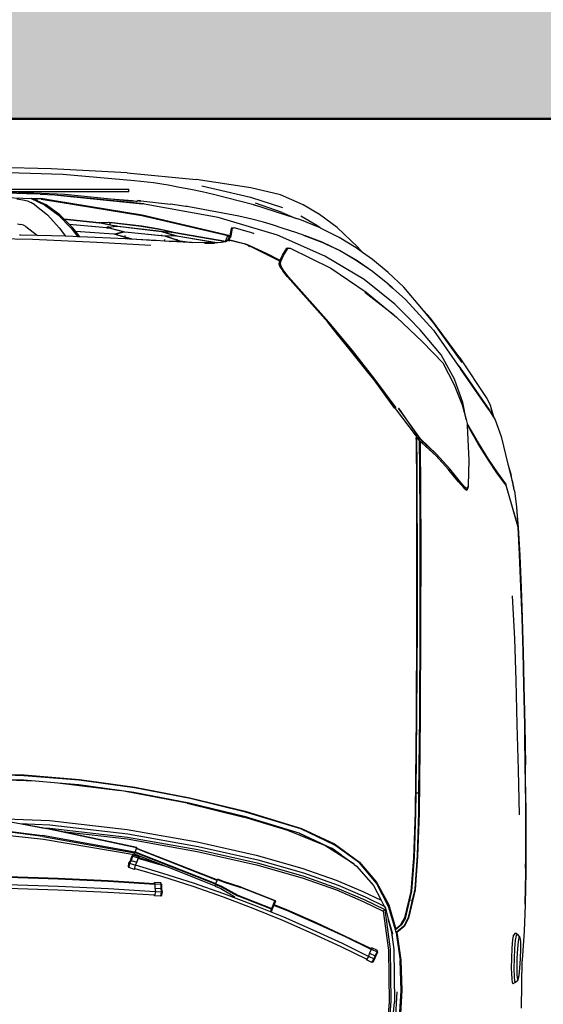
# Model space of a CAD drawing. Units: inches. Extents: x 22042254 to 25404563, y 17568978 to 17626777.
# Tile 34 of 45: x 22179853 to 22179890, y 17626332 to 17626402. Entities that reach past the tile are written whole.
import ezdxf

# ---------------------------------------------------------------- set-up
doc = ezdxf.new("R2010")
doc.units = ezdxf.units.IN
doc.header["$MEASUREMENT"] = 0
for name, color, linetype, lineweight in [('A-SITE-VEHI', 8, 'Continuous', 18), ('A-WALL-PATT', 244, 'Continuous', 13), ('walls', 252, 'Continuous', 50)]:
    doc.layers.add(name, color=color, linetype=linetype, lineweight=lineweight)
doc.layers.add('Edges', color=250, linetype='Continuous')

# ---------------------------------------------------------------- blocks, each defined once
blk = doc.blocks.new('Nissan Qashqai pl')
at = {"layer": 'Edges'}
for p, q in [((7.8676, 12.8123), (7.7998, 12.7928)), ((7.8012, 12.7929), (7.8681, 12.8121)), ((7.8363, 12.8097), (7.8676, 12.8123)), ((7.8381, 12.81), (7.87, 12.8126)), ((7.8676, 12.8123), (7.8681, 12.8121)), ((7.869, 12.8124), (7.8681, 12.8121)), ((7.9137, 12.815), (7.869, 12.8124)), ((7.87, 12.8126), (7.9151, 12.8152)), ((7.9658, 12.8172), (7.9137, 12.815)), ((7.9151, 12.8152), (7.9668, 12.8174)), ((8.016, 12.8189), (7.9658, 12.8172)), ((7.9668, 12.8174), (8.0168, 12.8191)), ((8.0713, 12.8205), (8.016, 12.8189)), ((8.0168, 12.8191), (8.0718, 12.8207)), ((8.1249, 12.8218), (8.0713, 12.8205)), ((8.0718, 12.8207), (8.1251, 12.822)), ((8.1901, 12.8232), (8.1249, 12.8218)), ((8.1251, 12.822), (8.1902, 12.8233)), ((8.1888, 12.8107), (8.2622, 12.8125)), ((8.2094, 12.8235), (8.1901, 12.8232)), ((8.1902, 12.8233), (8.2543, 12.8243)), ((8.2543, 12.8243), (8.2094, 12.8235)), ((8.2543, 12.8243), (8.2094, 12.8235)), ((8.2544, 12.8242), (8.2094, 12.8235)), ((8.2693, 12.8245), (8.2543, 12.8243)), ((8.3166, 12.8249), (8.2544, 12.8242)), ((8.2622, 12.8125), (8.3356, 12.8141)), ((8.3098, 12.825), (8.2693, 12.8245)), ((8.3159, 12.825), (8.2693, 12.8245)), ((8.3159, 12.825), (8.3098, 12.825)), ((8.3159, 12.825), (8.3163, 12.825)), ((8.3163, 12.825), (8.3657, 12.8252)), ((8.3163, 12.825), (8.3597, 12.8252)), ((8.3764, 12.8251), (8.3166, 12.8249)), ((8.3597, 12.8252), (8.3657, 12.8252)), ((8.3657, 12.8252), (8.3663, 12.8252)), ((8.3663, 12.8252), (8.3747, 12.8252)), ((8.3764, 12.8251), (8.3663, 12.8252)), ((8.3747, 12.8252), (8.3757, 12.8252)), ((8.3757, 12.8252), (8.4282, 12.8249)), ((8.4069, 12.8249), (8.3764, 12.8251)), ((8.4219, 12.8246), (8.4069, 12.8249)), ((8.4292, 12.8248), (8.4069, 12.8249)), ((8.4282, 12.8249), (8.4799, 12.8239)), ((8.4799, 12.8239), (8.4292, 12.8248)), ((8.4799, 12.8239), (8.4811, 12.8239)), ((8.4811, 12.8239), (8.5241, 12.8222)), ((8.5241, 12.8222), (8.5707, 12.8193)), ((8.5287, 12.8112), (8.5331, 12.815)), ((8.5347, 12.8159), (8.5331, 12.815)), ((8.5331, 12.815), (8.5346, 12.8138)), ((8.5346, 12.8138), (8.5406, 12.8125)), ((8.5407, 12.8167), (8.5347, 12.8159)), ((8.5406, 12.8125), (8.5526, 12.8114)), ((8.5527, 12.8169), (8.5407, 12.8167)), ((8.5682, 12.8164), (8.5527, 12.8169)), ((8.5837, 12.8154), (8.5682, 12.8164)), ((8.5707, 12.8193), (8.5719, 12.8193)), ((8.6489, 12.8179), (8.5719, 12.8193)), ((8.5958, 12.8141), (8.5837, 12.8154)), ((8.6018, 12.8129), (8.5958, 12.8141)), ((8.6017, 12.8114), (8.6032, 12.8121)), ((8.6032, 12.8121), (8.6018, 12.8129)), ((8.6073, 12.808), (8.6032, 12.8121)), ((7.7223, 12.7851), (7.7673, 12.7961)), ((7.7673, 12.7961), (7.8058, 12.8055)), ((7.7673, 12.7961), (7.7848, 12.8012)), ((7.7835, 12.8007), (7.7835, 12.8007)), ((7.8087, 12.8062), (7.7848, 12.8012)), ((7.7865, 12.8013), (7.7866, 12.8013)), ((7.7936, 12.8029), (7.7977, 12.8038)), ((7.8106, 12.8065), (7.8087, 12.8062)), ((7.8106, 12.8065), (7.8107, 12.8065)), ((7.8107, 12.8065), (7.8363, 12.8097)), ((7.8363, 12.8097), (7.8381, 12.81)), ((7.9803, 12.803), (8.05, 12.8066)), ((8.05, 12.8066), (8.1176, 12.8087)), ((8.1176, 12.8087), (8.1888, 12.8107)), ((8.5287, 12.8112), (8.5269, 12.8082)), ((8.5322, 12.8047), (8.5269, 12.8082)), ((8.5287, 12.8112), (8.531, 12.8095)), ((8.531, 12.8095), (8.5385, 12.8079)), ((8.5322, 12.8047), (8.5375, 12.8036)), ((8.5375, 12.8036), (8.5513, 12.8023)), ((8.5385, 12.8079), (8.5518, 12.8066)), ((8.5513, 12.8023), (8.5678, 12.8016)), ((8.5518, 12.8066), (8.568, 12.8059)), ((8.5526, 12.8114), (8.5681, 12.8107)), ((8.5678, 12.8016), (8.5844, 12.8014)), ((8.568, 12.8059), (8.5842, 12.8057)), ((8.5681, 12.8107), (8.5836, 12.8104)), ((8.5836, 12.8104), (8.5957, 12.8107)), ((8.5842, 12.8057), (8.5974, 12.8061)), ((8.5844, 12.8014), (8.5921, 12.8016)), ((8.5921, 12.8016), (8.6021, 12.8022)), ((8.5957, 12.8107), (8.6017, 12.8114)), ((8.5974, 12.8061), (8.6049, 12.8069)), ((8.6021, 12.8022), (8.6065, 12.8027)), ((8.6049, 12.8069), (8.6073, 12.808)), ((8.6065, 12.8027), (8.6093, 12.804)), ((8.6073, 12.808), (8.6093, 12.804)), ((7.6953, 12.7753), (7.7223, 12.7851)), ((7.7814, 12.7791), (7.7991, 12.7923)), ((7.7984, 12.7909), (7.7828, 12.7793)), ((7.7976, 12.792), (7.7991, 12.7923)), ((7.8007, 12.7926), (7.7984, 12.7909)), ((7.7991, 12.7923), (7.7998, 12.7928)), ((7.7995, 12.7924), (7.8007, 12.7926)), ((7.8012, 12.7929), (7.8007, 12.7926)), ((7.6799, 12.7658), (7.6125, 12.719)), ((7.6608, 12.7617), (7.6712, 12.7675)), ((7.6712, 12.7675), (7.6721, 12.7679)), ((7.6926, 12.7737), (7.6721, 12.7679)), ((7.6759, 12.7633), (7.6793, 12.7657)), ((7.6911, 12.7728), (7.6774, 12.7688)), ((7.6793, 12.7657), (7.6802, 12.766)), ((7.6799, 12.7658), (7.6802, 12.766)), ((7.6802, 12.766), (7.6809, 12.7664)), ((7.6809, 12.7664), (7.6911, 12.7728)), ((7.6911, 12.7728), (7.6926, 12.7737)), ((7.6926, 12.7737), (7.6953, 12.7753)), ((7.7325, 12.7476), (7.7591, 12.7641)), ((7.7606, 12.7644), (7.7341, 12.7478)), ((7.7591, 12.7641), (7.7814, 12.7791)), ((7.7828, 12.7793), (7.7606, 12.7644)), ((7.5946, 12.718), (7.6608, 12.7617)), ((7.6113, 12.7186), (7.6759, 12.7633)), ((7.7341, 12.7478), (7.7056, 12.7314)), ((7.7038, 12.731), (7.7325, 12.7476)), ((7.7048, 12.7302), (7.7608, 12.7329)), ((7.7608, 12.7329), (7.8014, 12.7318)), ((7.7688, 12.7328), (7.7688, 12.734)), ((7.5946, 12.718), (7.5304, 12.6704)), ((7.6024, 12.7221), (7.5387, 12.6759)), ((7.6051, 12.7139), (7.6113, 12.7186)), ((7.6051, 12.7139), (7.6111, 12.7181)), ((7.6118, 12.7186), (7.6111, 12.7181)), ((7.6125, 12.719), (7.6118, 12.7186)), ((7.667, 12.723), (7.6295, 12.7097)), ((7.6386, 12.7089), (7.6708, 12.7217)), ((7.6949, 12.7283), (7.667, 12.723)), ((7.6708, 12.7217), (7.6949, 12.7283)), ((7.6949, 12.7283), (7.701, 12.73)), ((7.701, 12.73), (7.7024, 12.7301)), ((7.7024, 12.7301), (7.7038, 12.731)), ((7.7024, 12.7301), (7.7034, 12.7301)), ((7.7056, 12.7314), (7.7034, 12.7301)), ((7.7034, 12.7301), (7.7048, 12.7302)), ((7.7058, 12.7308), (7.7048, 12.7302)), ((7.7938, 12.7171), (7.7748, 12.7018)), ((7.7959, 12.7161), (7.7772, 12.7011)), ((7.8045, 12.7263), (7.7938, 12.7171)), ((7.8062, 12.725), (7.7959, 12.7161)), ((7.8014, 12.7318), (7.8022, 12.7316)), ((7.8022, 12.7316), (7.8037, 12.7315)), ((7.8022, 12.7316), (7.8072, 12.73)), ((7.8037, 12.7315), (7.8096, 12.7294)), ((7.8072, 12.73), (7.8045, 12.7263)), ((7.8062, 12.725), (7.8087, 12.7283)), ((7.8066, 12.7254), (7.8062, 12.725)), ((7.8096, 12.7294), (7.8066, 12.7254)), ((7.8072, 12.73), (7.8087, 12.7283)), ((7.5501, 12.6757), (7.6051, 12.7139)), ((7.6295, 12.7097), (7.59, 12.6877)), ((7.6032, 12.6908), (7.6386, 12.7089)), ((7.7748, 12.7018), (7.7507, 12.6803)), ((7.7772, 12.7011), (7.776, 12.6999)), ((7.59, 12.6877), (7.5492, 12.654)), ((7.5687, 12.6579), (7.6032, 12.6908)), ((7.753, 12.6794), (7.776, 12.6999)), ((7.776, 12.6999), (7.7539, 12.68)), ((7.5501, 12.6757), (7.5001, 12.6302)), ((7.5387, 12.6759), (7.5184, 12.6591)), ((7.5184, 12.6591), (7.5304, 12.6704)), ((7.7261, 12.6543), (7.7507, 12.6803)), ((7.753, 12.6794), (7.7281, 12.6524)), ((7.7507, 12.6803), (7.7286, 12.6561)), ((7.7539, 12.68), (7.7324, 12.6565)), ((7.5184, 12.6591), (7.4801, 12.6274)), ((7.5289, 12.6158), (7.5687, 12.6579)), ((7.5492, 12.654), (7.531, 12.6359)), ((7.7261, 12.6543), (7.6762, 12.6186)), ((7.7281, 12.6524), (7.7232, 12.6486)), ((7.7267, 12.6539), (7.7233, 12.6514)), ((7.7286, 12.6561), (7.7267, 12.6539)), ((7.7299, 12.6537), (7.7281, 12.6524)), ((7.7281, 12.6524), (7.7349, 12.6524)), ((7.7324, 12.6565), (7.7299, 12.6537)), ((7.7299, 12.6537), (7.7334, 12.6537)), ((7.7334, 12.6537), (7.8083, 12.6544)), ((7.7349, 12.6524), (7.768, 12.6527)), ((7.768, 12.6527), (7.7692, 12.6527)), ((7.7692, 12.6527), (7.7844, 12.6528)), ((7.7844, 12.6528), (7.8078, 12.653)), ((7.8078, 12.653), (7.8233, 12.6531)), ((7.8083, 12.6544), (7.904, 12.6547)), ((7.8233, 12.6531), (7.9036, 12.6534)), ((7.9036, 12.6534), (8.0275, 12.6533)), ((7.904, 12.6547), (8.0276, 12.6545)), ((8.0275, 12.6533), (8.1755, 12.6527)), ((8.0276, 12.6545), (8.1753, 12.6539)), ((8.1753, 12.6539), (8.3324, 12.6521)), ((8.1755, 12.6527), (8.3005, 12.6514)), ((8.3324, 12.6521), (8.4022, 12.6498)), ((7.6762, 12.6186), (7.7233, 12.6514)), ((7.6771, 12.6135), (7.7215, 12.6473)), ((7.7215, 12.6473), (7.7221, 12.6478)), ((7.7232, 12.6486), (7.7221, 12.6478)), ((7.7245, 12.6486), (7.7232, 12.6486)), ((7.7261, 12.6476), (7.7238, 12.6476)), ((7.7294, 12.6487), (7.7245, 12.6486)), ((7.7279, 12.6477), (7.7261, 12.6476)), ((7.8048, 12.6483), (7.7279, 12.6477)), ((7.731, 12.6487), (7.7294, 12.6487)), ((7.764, 12.6489), (7.731, 12.6487)), ((7.7662, 12.6489), (7.764, 12.6489)), ((7.7811, 12.649), (7.7662, 12.6489)), ((7.7822, 12.649), (7.7811, 12.649)), ((7.8057, 12.6491), (7.7822, 12.649)), ((7.9014, 12.6487), (7.8048, 12.6483)), ((7.8233, 12.6492), (7.8057, 12.6491)), ((7.902, 12.6495), (7.8233, 12.6492)), ((8.0273, 12.6485), (7.9014, 12.6487)), ((8.0275, 12.6493), (7.902, 12.6495)), ((8.1753, 12.6479), (8.0273, 12.6485)), ((8.1754, 12.6487), (8.0275, 12.6493)), ((8.3318, 12.6462), (8.1753, 12.6479)), ((8.3002, 12.6474), (8.1754, 12.6487)), ((8.3005, 12.6514), (8.3002, 12.6474)), ((8.332, 12.6471), (8.3002, 12.6474)), ((8.3005, 12.6514), (8.3324, 12.651)), ((8.4049, 12.6437), (8.3318, 12.6462)), ((8.4042, 12.6447), (8.332, 12.6471)), ((8.3324, 12.651), (8.4014, 12.6488)), ((8.4014, 12.6488), (8.4559, 12.6451)), ((8.4022, 12.6498), (8.4571, 12.6459)), ((8.4588, 12.6405), (8.4042, 12.6447)), ((8.4595, 12.6395), (8.4049, 12.6437)), ((8.4559, 12.6451), (8.4736, 12.6409)), ((8.4571, 12.6459), (8.5029, 12.635)), ((8.4729, 12.6372), (8.4588, 12.6405)), ((8.5025, 12.6293), (8.4595, 12.6395)), ((8.4729, 12.6372), (8.4736, 12.6409)), ((8.5032, 12.6301), (8.4729, 12.6372)), ((8.4736, 12.6409), (8.5018, 12.6344)), ((7.4801, 12.6274), (7.4565, 12.6023)), ((7.4827, 12.6103), (7.5001, 12.6302)), ((7.531, 12.6359), (7.5081, 12.6131)), ((7.531, 12.6359), (7.5301, 12.6353)), ((8.5018, 12.6344), (8.5155, 12.6274)), ((8.5125, 12.6231), (8.5025, 12.6293)), ((8.5029, 12.635), (8.5163, 12.6279)), ((8.5132, 12.624), (8.5032, 12.6301)), ((8.5177, 12.617), (8.5125, 12.6231)), ((8.5132, 12.624), (8.5216, 12.6139)), ((8.5155, 12.6274), (8.5258, 12.6151)), ((8.5163, 12.6279), (8.5237, 12.6189)), ((8.5294, 12.6167), (8.5706, 12.6226)), ((8.5304, 12.6157), (8.5715, 12.6215)), ((8.5706, 12.6226), (8.6197, 12.6241)), ((8.6203, 12.6229), (8.5715, 12.6215)), ((8.6197, 12.6241), (8.6683, 12.6215)), ((8.6203, 12.6229), (8.6204, 12.6229)), ((8.6721, 12.6201), (8.6204, 12.6229)), ((7.5081, 12.6131), (7.4679, 12.5634)), ((7.4744, 12.6015), (7.4804, 12.6079)), ((7.4762, 12.6028), (7.478, 12.6049)), ((7.4804, 12.6079), (7.478, 12.6049)), ((7.478, 12.6049), (7.479, 12.6061)), ((7.479, 12.6061), (7.4815, 12.6089)), ((7.479, 12.6061), (7.4801, 12.6074)), ((7.4801, 12.6074), (7.4804, 12.6079)), ((7.4804, 12.6079), (7.4807, 12.6082)), ((7.4804, 12.6079), (7.4804, 12.6079)), ((7.4807, 12.6082), (7.4821, 12.6097)), ((7.4815, 12.6089), (7.4821, 12.6097)), ((7.4821, 12.6097), (7.4827, 12.6103)), ((7.4882, 12.5645), (7.5243, 12.6101)), ((7.4884, 12.5664), (7.5289, 12.6158)), ((7.5243, 12.6101), (7.5286, 12.6146)), ((7.676, 12.6152), (7.6296, 12.5803)), ((7.6769, 12.6129), (7.6306, 12.5791)), ((8.4814, 12.6029), (8.5166, 12.6135)), ((8.5216, 12.6139), (8.4838, 12.6027)), ((8.4889, 12.5969), (8.5531, 12.6055)), ((8.5039, 12.6023), (8.528, 12.6088)), ((8.5216, 12.6068), (8.5039, 12.6023)), ((8.5166, 12.6135), (8.5197, 12.6145)), ((8.5197, 12.6145), (8.5177, 12.617)), ((8.5197, 12.6145), (8.5216, 12.6139)), ((8.5258, 12.6151), (8.5216, 12.6139)), ((8.5216, 12.6068), (8.5538, 12.6111)), ((8.5301, 12.609), (8.5216, 12.6068)), ((8.5237, 12.6189), (8.5259, 12.6162)), ((8.5259, 12.6162), (8.5258, 12.6151)), ((8.5258, 12.6151), (8.5304, 12.6157)), ((8.5259, 12.6162), (8.5294, 12.6167)), ((8.5304, 12.6157), (8.5304, 12.6157)), ((8.5531, 12.6055), (8.6375, 12.6066)), ((8.5538, 12.6111), (8.6387, 12.6123)), ((8.622, 12.6161), (8.6699, 12.6132)), ((8.6375, 12.6066), (8.7481, 12.5968)), ((8.6721, 12.6093), (8.6387, 12.6123)), ((7.4565, 12.6023), (7.4354, 12.5766)), ((7.4542, 12.5765), (7.4744, 12.6015)), ((7.475, 12.6016), (7.4549, 12.5767)), ((7.4762, 12.6028), (7.475, 12.6016)), ((7.4752, 12.6016), (7.4762, 12.6028)), ((8.4444, 12.5834), (8.4814, 12.6029)), ((8.4838, 12.6027), (8.4462, 12.5833)), ((8.4499, 12.5782), (8.4737, 12.5908)), ((8.4594, 12.5611), (8.4737, 12.5908)), ((8.468, 12.5648), (8.4831, 12.5957)), ((8.4725, 12.563), (8.4889, 12.5969)), ((8.4737, 12.5908), (8.4831, 12.5957)), ((8.4756, 12.5615), (8.4914, 12.5942)), ((8.4831, 12.5957), (8.4867, 12.5977)), ((8.4867, 12.5977), (8.5039, 12.6023)), ((8.4914, 12.5942), (8.4889, 12.5969)), ((8.4914, 12.5942), (8.5544, 12.6026)), ((8.5544, 12.6026), (8.6386, 12.6037)), ((8.6386, 12.6037), (8.7491, 12.594)), ((7.4354, 12.5766), (7.4239, 12.5604)), ((7.4363, 12.5502), (7.4542, 12.5765)), ((7.4549, 12.5767), (7.4369, 12.5504)), ((7.6296, 12.5803), (7.5827, 12.5441)), ((7.6301, 12.5787), (7.618, 12.5691)), ((7.6306, 12.5791), (7.6301, 12.5787)), ((8.4122, 12.5558), (8.4444, 12.5834)), ((8.4462, 12.5833), (8.4134, 12.5554)), ((8.4183, 12.5508), (8.4499, 12.5782)), ((8.5527, 12.5749), (8.5323, 12.5332)), ((8.5537, 12.5747), (8.5332, 12.5329)), ((8.5554, 12.5847), (8.551, 12.5757)), ((8.5527, 12.5749), (8.551, 12.5757)), ((8.551, 12.5757), (8.5528, 12.5751)), ((8.5528, 12.5751), (8.5527, 12.5749)), ((8.5528, 12.5751), (8.5529, 12.5751)), ((8.5529, 12.5751), (8.5572, 12.5841)), ((8.5529, 12.5751), (8.5537, 12.5747)), ((8.5537, 12.5747), (8.5595, 12.572)), ((8.5574, 12.5849), (8.5554, 12.5847)), ((8.5572, 12.5841), (8.5554, 12.5847)), ((8.5639, 12.581), (8.5572, 12.5841)), ((8.5574, 12.5849), (8.5584, 12.5846)), ((8.5582, 12.5845), (8.5574, 12.5849)), ((8.5584, 12.5846), (8.5649, 12.5816)), ((8.5595, 12.572), (8.5639, 12.581)), ((8.5687, 12.5791), (8.5639, 12.581)), ((8.5644, 12.5701), (8.5687, 12.5791)), ((8.5649, 12.5816), (8.5693, 12.5799)), ((8.5687, 12.5791), (8.5693, 12.5799)), ((8.5749, 12.5757), (8.5687, 12.5791)), ((8.5693, 12.5799), (8.5739, 12.5774)), ((8.5749, 12.5757), (8.5705, 12.5668)), ((8.5739, 12.5774), (8.5749, 12.5757)), ((7.4239, 12.5604), (7.4147, 12.5524)), ((7.4239, 12.5604), (7.4166, 12.5503)), ((7.4679, 12.5634), (7.4302, 12.4993)), ((7.4498, 12.5093), (7.4884, 12.5664)), ((7.618, 12.5691), (7.5829, 12.5411)), ((7.618, 12.5691), (7.584, 12.5429)), ((8.4411, 12.5178), (8.4594, 12.5611)), ((8.4493, 12.5212), (8.468, 12.5648)), ((8.454, 12.5196), (8.4725, 12.563)), ((8.4571, 12.5184), (8.4756, 12.5615)), ((8.5647, 12.57), (8.5441, 12.5279)), ((8.5487, 12.5256), (8.5692, 12.5674)), ((8.5595, 12.572), (8.5644, 12.5701)), ((8.5644, 12.5701), (8.5647, 12.57)), ((8.5647, 12.57), (8.5692, 12.5675)), ((8.5692, 12.5674), (8.5692, 12.5675)), ((8.5692, 12.5675), (8.5705, 12.5668)), ((8.5705, 12.5668), (8.5692, 12.5674)), ((7.4147, 12.5524), (7.3837, 12.5197)), ((7.4166, 12.5503), (7.3997, 12.5227)), ((7.4205, 12.5229), (7.4363, 12.5502)), ((7.4369, 12.5504), (7.4211, 12.5232)), ((7.5827, 12.5441), (7.5369, 12.5057)), ((7.584, 12.5429), (7.5568, 12.5201)), ((7.5829, 12.5411), (7.5568, 12.5201)), ((8.3826, 12.5151), (8.4122, 12.5558)), ((8.4134, 12.5554), (8.3844, 12.5157)), ((8.4154, 12.5468), (8.3852, 12.4994)), ((8.3901, 12.5113), (8.4154, 12.5468)), ((8.4011, 12.5269), (8.4154, 12.5468)), ((8.4156, 12.547), (8.4154, 12.5468)), ((8.4156, 12.547), (8.4183, 12.5508)), ((8.4011, 12.5269), (8.3901, 12.5113)), ((8.3904, 12.512), (8.4011, 12.5269)), ((8.5323, 12.5332), (8.5103, 12.4859)), ((8.5332, 12.5329), (8.5112, 12.4856)), ((8.5441, 12.5279), (8.5222, 12.4807)), ((8.5269, 12.4785), (8.5487, 12.5256)), ((7.3837, 12.5197), (7.3624, 12.4907)), ((7.3997, 12.5227), (7.3845, 12.4925)), ((7.4071, 12.4948), (7.4205, 12.5229)), ((7.4211, 12.5232), (7.4078, 12.4951)), ((7.4172, 12.4431), (7.4498, 12.5093)), ((7.5568, 12.5201), (7.5371, 12.5042)), ((8.3573, 12.4618), (8.3826, 12.5151)), ((8.3844, 12.5157), (8.3582, 12.4606)), ((8.3646, 12.4572), (8.39, 12.5111)), ((8.3648, 12.4579), (8.39, 12.5111)), ((8.39, 12.5111), (8.3852, 12.4994)), ((8.39, 12.5111), (8.3901, 12.5113)), ((8.3901, 12.5113), (8.3904, 12.512)), ((8.4217, 12.4622), (8.4411, 12.5178)), ((8.4296, 12.4651), (8.4493, 12.5212)), ((8.4343, 12.4637), (8.454, 12.5196)), ((8.4375, 12.4627), (8.4571, 12.5184)), ((7.3962, 12.466), (7.4071, 12.4948)), ((7.4302, 12.4993), (7.3963, 12.4227)), ((7.4078, 12.4951), (7.3969, 12.4665)), ((7.5369, 12.5057), (7.4635, 12.4408)), ((7.4638, 12.439), (7.5371, 12.5042)), ((8.3852, 12.4994), (8.3608, 12.4393)), ((7.3624, 12.4907), (7.347, 12.4644)), ((7.3805, 12.4866), (7.3655, 12.4604)), ((7.3843, 12.492), (7.3707, 12.4592)), ((7.3843, 12.492), (7.3805, 12.4866)), ((7.3845, 12.4925), (7.3843, 12.492)), ((8.5103, 12.4859), (8.4895, 12.4381)), ((8.5112, 12.4856), (8.4904, 12.4377)), ((8.5222, 12.4807), (8.5014, 12.4329)), ((8.5062, 12.431), (8.5269, 12.4785)), ((7.347, 12.4644), (7.3309, 12.4276)), ((7.3951, 12.462), (7.3938, 12.4583)), ((7.3965, 12.4655), (7.3951, 12.462)), ((7.3965, 12.4655), (7.3962, 12.466)), ((7.3969, 12.4665), (7.3965, 12.4655)), ((7.3968, 12.4649), (7.3967, 12.4651)), ((8.3296, 12.3703), (8.3573, 12.4618)), ((8.4009, 12.3883), (8.4217, 12.4622)), ((8.4084, 12.3907), (8.4296, 12.4651)), ((8.4133, 12.3896), (8.4343, 12.4637)), ((8.4165, 12.3888), (8.4375, 12.4627)), ((7.3688, 12.4532), (7.3467, 12.3846)), ((7.3596, 12.4302), (7.3688, 12.4532)), ((7.3707, 12.4592), (7.3688, 12.4532)), ((7.3925, 12.4542), (7.3845, 12.4306)), ((7.3938, 12.4583), (7.3925, 12.4542)), ((8.3582, 12.4606), (8.3311, 12.3708)), ((8.3377, 12.3689), (8.3646, 12.4572)), ((8.3646, 12.4572), (8.3648, 12.4579)), ((8.3648, 12.4579), (8.3648, 12.4579)), ((7.3345, 12.3793), (7.3514, 12.4308)), ((7.3596, 12.4302), (7.344, 12.3869)), ((7.3845, 12.4306), (7.3799, 12.4164)), ((7.4167, 12.4393), (7.4169, 12.4406)), ((7.4167, 12.4393), (7.4172, 12.4395)), ((7.417, 12.4377), (7.4167, 12.4393)), ((7.4169, 12.4412), (7.4172, 12.4431)), ((7.4169, 12.4406), (7.4172, 12.4423)), ((7.4169, 12.4406), (7.4169, 12.4412)), ((7.4169, 12.4398), (7.4169, 12.4406)), ((7.4282, 12.4328), (7.4169, 12.4398)), ((7.4172, 12.4395), (7.4169, 12.4398)), ((7.4283, 12.4307), (7.417, 12.4377)), ((7.4172, 12.4423), (7.4174, 12.4429)), ((7.4183, 12.4382), (7.4172, 12.4395)), ((7.4175, 12.4429), (7.4174, 12.4429)), ((7.4183, 12.4382), (7.4296, 12.4312)), ((7.4387, 12.428), (7.4282, 12.4328)), ((7.4359, 12.4272), (7.4283, 12.4307)), ((7.4383, 12.4272), (7.4296, 12.4312)), ((7.4479, 12.4293), (7.4431, 12.4276)), ((7.4477, 12.427), (7.4541, 12.4313)), ((7.4541, 12.4333), (7.4479, 12.4293)), ((7.4635, 12.4408), (7.4541, 12.4333)), ((7.4638, 12.439), (7.4541, 12.4313)), ((8.3608, 12.4393), (8.3392, 12.3684)), ((8.3608, 12.4393), (8.3608, 12.4393)), ((8.4895, 12.4381), (8.4811, 12.4174)), ((8.5014, 12.4329), (8.4817, 12.3847)), ((8.4904, 12.4377), (8.482, 12.4171)), ((8.4866, 12.3829), (8.5062, 12.431)), ((7.3309, 12.4276), (7.3193, 12.3797)), ((7.3963, 12.4227), (7.3676, 12.3269)), ((7.3799, 12.4164), (7.375, 12.4)), ((7.4255, 12.4044), (7.4367, 12.4268)), ((7.4365, 12.4235), (7.4267, 12.4041)), ((7.4367, 12.4268), (7.4359, 12.4272)), ((7.4378, 12.4261), (7.4365, 12.4235)), ((7.4365, 12.4235), (7.4365, 12.4235)), ((7.4367, 12.4268), (7.4383, 12.4272)), ((7.4379, 12.4263), (7.4378, 12.4261)), ((7.4379, 12.4263), (7.4383, 12.4272)), ((7.4379, 12.4263), (7.4389, 12.4269)), ((7.4384, 12.426), (7.4379, 12.4263)), ((7.4384, 12.426), (7.438, 12.4251)), ((7.4383, 12.4272), (7.4389, 12.4269)), ((7.4389, 12.4269), (7.4384, 12.426)), ((7.4387, 12.4259), (7.4384, 12.426)), ((7.4431, 12.4276), (7.4387, 12.428)), ((7.443, 12.4254), (7.4387, 12.4259)), ((7.44, 12.4264), (7.4389, 12.4269)), ((7.44, 12.4264), (7.4442, 12.4258)), ((7.4477, 12.427), (7.443, 12.4254)), ((7.4442, 12.4258), (7.4477, 12.427)), ((8.4526, 12.3639), (8.4742, 12.4188)), ((8.4747, 12.4185), (8.4532, 12.3636)), ((8.4654, 12.3587), (8.4869, 12.4136)), ((8.4881, 12.4131), (8.4666, 12.3582)), ((8.4742, 12.4188), (8.4754, 12.4193)), ((8.4747, 12.4185), (8.4742, 12.4188)), ((8.4754, 12.4193), (8.4747, 12.4185)), ((8.4869, 12.4136), (8.4747, 12.4185)), ((8.4754, 12.4193), (8.4876, 12.4144)), ((8.4791, 12.4183), (8.4754, 12.4193)), ((8.4811, 12.4174), (8.4791, 12.4183)), ((8.482, 12.4171), (8.4811, 12.4174)), ((8.4912, 12.4133), (8.482, 12.4171)), ((8.4869, 12.4136), (8.4876, 12.4144)), ((8.4881, 12.4131), (8.4869, 12.4136)), ((8.4876, 12.4144), (8.4912, 12.4133)), ((8.4876, 12.4144), (8.4881, 12.4131)), ((8.4914, 12.4121), (8.4881, 12.4131)), ((8.4913, 12.4133), (8.4912, 12.4133)), ((8.4913, 12.4132), (8.4913, 12.4133)), ((7.375, 12.4), (7.3699, 12.3813)), ((7.4131, 12.3783), (7.4255, 12.4044)), ((7.4267, 12.4041), (7.4139, 12.3778)), ((7.3467, 12.3846), (7.33, 12.3192)), ((7.3467, 12.3846), (7.3489, 12.3925)), ((7.3699, 12.3813), (7.3653, 12.3604)), ((7.3925, 12.3813), (7.3914, 12.3775)), ((7.3937, 12.3851), (7.3925, 12.3813)), ((8.3792, 12.2926), (8.4009, 12.3883)), ((8.3864, 12.2945), (8.4084, 12.3907)), ((8.3913, 12.2935), (8.4133, 12.3896)), ((8.3945, 12.2929), (8.4165, 12.3888)), ((8.4817, 12.3847), (8.4633, 12.3359)), ((8.4683, 12.3345), (8.4866, 12.3829)), ((7.3193, 12.3797), (7.3059, 12.291)), ((7.3161, 12.3001), (7.3345, 12.3793)), ((7.3913, 12.3774), (7.3844, 12.3526)), ((7.3913, 12.3774), (7.3914, 12.3775)), ((7.4033, 12.3435), (7.4101, 12.3708)), ((7.4108, 12.3703), (7.4042, 12.3435)), ((7.4101, 12.3708), (7.4115, 12.3746)), ((7.4122, 12.3742), (7.4108, 12.3703)), ((7.4115, 12.3746), (7.4131, 12.3783)), ((7.4139, 12.3778), (7.4122, 12.3742)), ((7.4133, 12.3759), (7.4142, 12.3776)), ((8.3076, 12.281), (8.3296, 12.3703)), ((8.3311, 12.3708), (8.3089, 12.2811)), ((8.3157, 12.2795), (8.3377, 12.3689)), ((8.3166, 12.2767), (8.3392, 12.3684)), ((7.3653, 12.3604), (7.3497, 12.2767)), ((7.3841, 12.3485), (7.3844, 12.3526)), ((7.3846, 12.3495), (7.3841, 12.3485)), ((7.3846, 12.3495), (7.3976, 12.347)), ((8.4526, 12.3639), (8.4434, 12.3353)), ((8.4439, 12.335), (8.4532, 12.3636)), ((8.4509, 12.3322), (8.4654, 12.3587)), ((8.4521, 12.3317), (8.4666, 12.3582)), ((8.4547, 12.3309), (8.4682, 12.3538)), ((7.3971, 12.3461), (7.3635, 12.2033)), ((7.364, 12.2029), (7.3968, 12.3424)), ((7.3841, 12.3485), (7.3853, 12.3483)), ((7.3971, 12.3461), (7.3853, 12.3483)), ((7.3916, 12.2547), (7.4062, 12.3389)), ((7.4065, 12.3392), (7.3917, 12.2547)), ((7.3968, 12.3424), (7.398, 12.3449)), ((7.4046, 12.3389), (7.3968, 12.3424)), ((7.3983, 12.3458), (7.3971, 12.3461)), ((7.3976, 12.347), (7.4026, 12.3439)), ((7.398, 12.3449), (7.3999, 12.344)), ((7.398, 12.3449), (7.4012, 12.3441)), ((7.4012, 12.3441), (7.3983, 12.3458)), ((7.3999, 12.344), (7.4051, 12.3415)), ((7.3999, 12.344), (7.4048, 12.3417)), ((7.4033, 12.3427), (7.4012, 12.3441)), ((7.4012, 12.3441), (7.4015, 12.344)), ((7.4015, 12.344), (7.4028, 12.3437)), ((7.4026, 12.3439), (7.4033, 12.3435)), ((7.4033, 12.3435), (7.4042, 12.3422)), ((7.4042, 12.3422), (7.4033, 12.3427)), ((7.4042, 12.3435), (7.404, 12.3429)), ((7.404, 12.3429), (7.4043, 12.3428)), ((7.404, 12.3429), (7.4043, 12.3425)), ((7.4041, 12.3435), (7.4042, 12.3435)), ((7.4042, 12.3435), (7.4045, 12.3434)), ((7.4042, 12.3422), (7.4043, 12.3425)), ((7.4044, 12.3422), (7.4042, 12.3422)), ((7.4043, 12.3428), (7.4045, 12.3434)), ((7.4043, 12.3428), (7.4046, 12.3425)), ((7.4043, 12.3425), (7.4043, 12.3428)), ((7.4043, 12.3425), (7.4044, 12.3422)), ((7.4044, 12.3422), (7.4046, 12.3419)), ((7.4046, 12.3422), (7.4044, 12.3422)), ((7.4045, 12.3434), (7.405, 12.3456)), ((7.4045, 12.3434), (7.4048, 12.3433)), ((7.4046, 12.3425), (7.4047, 12.3424)), ((7.4047, 12.3424), (7.4046, 12.3422)), ((7.4046, 12.3422), (7.4046, 12.3419)), ((7.4048, 12.3422), (7.4046, 12.3422)), ((7.4046, 12.3419), (7.405, 12.3419)), ((7.4048, 12.3417), (7.4046, 12.3419)), ((7.4046, 12.3389), (7.4062, 12.3389)), ((7.4047, 12.3424), (7.4048, 12.3422)), ((7.4048, 12.3422), (7.405, 12.3419)), ((7.4048, 12.3417), (7.4052, 12.3416)), ((7.4051, 12.3415), (7.4048, 12.3417)), ((7.405, 12.3419), (7.4052, 12.3416)), ((7.4051, 12.3415), (7.4052, 12.3415)), ((7.4052, 12.3416), (7.4052, 12.3415)), ((7.4052, 12.3415), (7.4063, 12.3395)), ((7.4062, 12.3389), (7.4063, 12.3395)), ((7.4063, 12.3395), (7.4065, 12.3392)), ((7.4065, 12.3392), (7.4066, 12.3389)), ((7.4066, 12.3389), (7.408, 12.3313)), ((8.4434, 12.3353), (8.4397, 12.326)), ((8.4403, 12.3257), (8.4439, 12.335)), ((8.4633, 12.3359), (8.4461, 12.2868)), ((8.4512, 12.2856), (8.4683, 12.3345)), ((7.33, 12.3192), (7.3261, 12.3009)), ((7.3676, 12.3269), (7.3455, 12.2042)), ((7.3971, 12.2599), (7.4083, 12.3258)), ((7.4084, 12.3244), (7.3975, 12.2599)), ((7.408, 12.3313), (7.4083, 12.3258)), ((7.4083, 12.3258), (7.4084, 12.3244)), ((7.4084, 12.3244), (7.4087, 12.3195)), ((7.4087, 12.3195), (7.4087, 12.3037)), ((7.4092, 12.3184), (7.4091, 12.3206)), ((7.4092, 12.305), (7.4092, 12.3184)), ((8.3894, 12.1944), (8.4409, 12.3255)), ((8.4415, 12.3252), (8.3899, 12.1941)), ((8.3951, 12.192), (8.4467, 12.3231)), ((8.4479, 12.3226), (8.3963, 12.1915)), ((8.4209, 12.2475), (8.4502, 12.3219)), ((8.4403, 12.3257), (8.4397, 12.326)), ((8.4409, 12.3255), (8.4403, 12.3257)), ((8.4415, 12.3252), (8.4409, 12.3255)), ((8.4467, 12.3231), (8.4415, 12.3252)), ((8.4472, 12.3229), (8.4467, 12.3231)), ((8.4472, 12.3229), (8.4509, 12.3322)), ((8.4479, 12.3226), (8.4472, 12.3229)), ((8.4484, 12.3224), (8.4479, 12.3226)), ((8.4484, 12.3224), (8.4521, 12.3317)), ((8.4502, 12.3219), (8.4484, 12.3224)), ((8.4511, 12.3216), (8.4502, 12.3219)), ((8.4511, 12.3216), (8.4547, 12.3309)), ((7.4087, 12.3037), (7.4081, 12.2848)), ((7.2951, 12.1791), (7.3059, 12.291)), ((7.3261, 12.3009), (7.3223, 12.2825)), ((8.3593, 12.1791), (8.3792, 12.2926)), ((8.3662, 12.1803), (8.3864, 12.2945)), ((8.3713, 12.1796), (8.3913, 12.2935)), ((8.3745, 12.1792), (8.3945, 12.2929)), ((8.4461, 12.2868), (8.4302, 12.2373)), ((8.4353, 12.2363), (8.4512, 12.2856)), ((7.3223, 12.2825), (7.3186, 12.2641)), ((7.3494, 12.2741), (7.3457, 12.2495)), ((7.3498, 12.2768), (7.3494, 12.2741)), ((7.3497, 12.2767), (7.3494, 12.2741)), ((7.4054, 12.2651), (7.4081, 12.2848)), ((7.4079, 12.2798), (7.4059, 12.2651)), ((7.4079, 12.2798), (7.4069, 12.2598)), ((7.4081, 12.2838), (7.4079, 12.2798)), ((7.4081, 12.2848), (7.4081, 12.2838)), ((8.2905, 12.1918), (8.3076, 12.281)), ((8.3089, 12.2811), (8.2916, 12.1913)), ((8.3166, 12.2767), (8.296, 12.168)), ((8.2985, 12.1901), (8.3157, 12.2795)), ((7.3186, 12.2641), (7.3149, 12.2457)), ((7.3908, 12.2366), (7.3965, 12.256)), ((7.391, 12.2387), (7.3967, 12.2579)), ((7.3912, 12.2527), (7.3916, 12.2547)), ((7.3917, 12.2547), (7.3914, 12.2527)), ((7.3969, 12.257), (7.3965, 12.256)), ((7.3967, 12.2579), (7.3971, 12.2599)), ((7.3968, 12.2559), (7.3969, 12.257)), ((7.3972, 12.2421), (7.3968, 12.2559)), ((7.3975, 12.2599), (7.3973, 12.258)), ((7.3973, 12.258), (7.3977, 12.2439)), ((7.4048, 12.2612), (7.3982, 12.2419)), ((7.3983, 12.244), (7.4038, 12.2599)), ((7.4028, 12.2599), (7.4038, 12.2599)), ((7.4038, 12.2599), (7.4049, 12.2631)), ((7.4053, 12.2622), (7.4048, 12.2612)), ((7.4049, 12.2631), (7.4054, 12.2651)), ((7.4053, 12.2612), (7.4053, 12.2622)), ((7.4061, 12.2473), (7.4053, 12.2612)), ((7.4059, 12.2618), (7.4056, 12.2621)), ((7.4059, 12.2651), (7.4058, 12.2632)), ((7.4058, 12.2632), (7.4059, 12.2618)), ((7.4059, 12.2618), (7.4064, 12.2523)), ((7.4069, 12.2598), (7.4064, 12.2523)), ((7.3149, 12.2457), (7.3113, 12.2217)), ((7.3407, 12.2016), (7.3457, 12.2495)), ((7.3909, 12.2508), (7.3864, 12.231)), ((7.3869, 12.2347), (7.3912, 12.2527)), ((7.3901, 12.2368), (7.391, 12.2507)), ((7.3914, 12.2527), (7.3906, 12.2386)), ((7.3906, 12.2386), (7.3907, 12.2376)), ((7.3907, 12.2376), (7.391, 12.2387)), ((7.3911, 12.2518), (7.3909, 12.2508)), ((7.391, 12.2507), (7.3911, 12.2518)), ((7.3912, 12.2517), (7.3911, 12.2518)), ((7.3977, 12.24), (7.3911, 12.1755)), ((7.3966, 12.2348), (7.3972, 12.24)), ((7.3972, 12.24), (7.3972, 12.2421)), ((7.3977, 12.2439), (7.398, 12.2429)), ((7.3982, 12.2419), (7.3977, 12.24)), ((7.398, 12.2429), (7.3983, 12.244)), ((7.4032, 12.24), (7.4057, 12.24)), ((7.4057, 12.24), (7.4048, 12.2262)), ((7.4061, 12.2472), (7.4057, 12.24)), ((7.4064, 12.2523), (7.4061, 12.2473)), ((7.4061, 12.2472), (7.4061, 12.2473)), ((8.4191, 12.2418), (8.4061, 12.1973)), ((8.4163, 12.2359), (8.4209, 12.2475)), ((8.4302, 12.2373), (8.4171, 12.1926)), ((8.4209, 12.2475), (8.4191, 12.2418)), ((7.3113, 12.2217), (7.3078, 12.191)), ((7.3813, 12.2021), (7.3869, 12.2347)), ((7.3815, 12.1638), (7.3899, 12.2348)), ((7.3864, 12.231), (7.3815, 12.2029)), ((7.3903, 12.2347), (7.382, 12.1639)), ((7.3899, 12.2348), (7.3901, 12.2368)), ((7.3908, 12.2366), (7.3903, 12.2347)), ((7.3905, 12.1754), (7.3966, 12.2347)), ((7.3957, 12.2348), (7.3966, 12.2348)), ((7.3957, 12.2347), (7.3966, 12.2347)), ((7.3966, 12.2347), (7.3966, 12.2348)), ((7.4022, 12.187), (7.4048, 12.2262)), ((7.4048, 12.2262), (7.4023, 12.1836)), ((8.3986, 12.1908), (8.4163, 12.2359)), ((8.4163, 12.2359), (8.4052, 12.1979)), ((8.4224, 12.1919), (8.4353, 12.2363)), ((8.4471, 12.2238), (8.4425, 12.1485)), ((8.448, 12.2241), (8.4435, 12.1487)), ((8.4457, 12.2337), (8.4452, 12.2238)), ((8.4452, 12.2238), (8.4471, 12.2242)), ((8.4471, 12.2238), (8.4452, 12.2238)), ((8.4475, 12.2348), (8.4457, 12.2337)), ((8.4476, 12.2341), (8.4457, 12.2337)), ((8.4471, 12.2242), (8.4476, 12.2341)), ((8.4471, 12.2242), (8.4544, 12.2242)), ((8.4471, 12.2239), (8.4471, 12.2238)), ((8.4475, 12.2348), (8.4484, 12.235)), ((8.4555, 12.2348), (8.4475, 12.2348)), ((8.4549, 12.2341), (8.4476, 12.2341)), ((8.4484, 12.235), (8.4557, 12.235)), ((8.4544, 12.2242), (8.4549, 12.2341)), ((8.4544, 12.2242), (8.4595, 12.2249)), ((8.46, 12.2348), (8.4549, 12.2341)), ((8.4601, 12.2247), (8.4555, 12.1488)), ((8.4557, 12.235), (8.4603, 12.2357)), ((8.4595, 12.2249), (8.46, 12.2348)), ((8.4595, 12.2249), (8.4666, 12.2237)), ((8.46, 12.2348), (8.4603, 12.2357)), ((8.4671, 12.2337), (8.46, 12.2348)), ((8.4603, 12.2357), (8.4655, 12.2348)), ((8.4607, 12.1481), (8.4652, 12.2237)), ((8.4652, 12.2237), (8.4652, 12.2238)), ((8.4666, 12.2237), (8.4652, 12.2237)), ((8.4655, 12.2348), (8.4671, 12.2337)), ((8.4671, 12.2337), (8.4666, 12.2237)), ((7.3455, 12.2062), (7.3317, 12.0717)), ((7.4072, 12.1299), (7.4124, 12.2176)), ((7.3078, 12.191), (7.298, 12.075)), ((7.3317, 12.0717), (7.3455, 12.2042)), ((7.3407, 12.2016), (7.34, 12.1962)), ((7.34, 12.1962), (7.3401, 12.1962)), ((7.3401, 12.1962), (7.341, 12.1962)), ((7.3403, 12.1981), (7.3407, 12.2016)), ((7.3635, 12.2033), (7.3405, 12.0616)), ((7.3413, 12.1933), (7.3407, 12.1879)), ((7.341, 12.1962), (7.3414, 12.1962)), ((7.341, 12.1962), (7.341, 12.1962)), ((7.3414, 12.1962), (7.341, 12.1962)), ((7.341, 12.1962), (7.3413, 12.1933)), ((7.3413, 12.1931), (7.341, 12.1848)), ((7.3415, 12.1954), (7.3413, 12.1933)), ((7.3413, 12.1933), (7.3413, 12.1931)), ((7.3426, 12.0707), (7.364, 12.2029)), ((7.375, 12.1484), (7.3813, 12.2021)), ((7.3815, 12.2029), (7.3756, 12.1509)), ((8.2781, 12.1018), (8.2905, 12.1918)), ((8.2916, 12.1913), (8.2793, 12.1016)), ((8.2862, 12.1008), (8.2985, 12.1901)), ((8.3887, 12.1946), (8.3575, 12.0475)), ((8.3882, 12.1948), (8.3618, 12.07)), ((8.3957, 12.1917), (8.3688, 12.0419)), ((8.3702, 12.0427), (8.3969, 12.1913)), ((8.3746, 12.0435), (8.3995, 12.1905)), ((8.3887, 12.1946), (8.3882, 12.1948)), ((8.3882, 12.1948), (8.3894, 12.1944)), ((8.3894, 12.1944), (8.3887, 12.1946)), ((8.3894, 12.1944), (8.3894, 12.1944)), ((8.3894, 12.1944), (8.3899, 12.1941)), ((8.3899, 12.1941), (8.3951, 12.192)), ((8.3951, 12.192), (8.3963, 12.1915)), ((8.3957, 12.1917), (8.3951, 12.192)), ((8.3969, 12.1913), (8.3957, 12.1917)), ((8.3963, 12.1915), (8.3986, 12.1908)), ((8.3995, 12.1905), (8.3969, 12.1913)), ((8.3995, 12.1905), (8.3986, 12.1908)), ((8.4035, 12.1986), (8.4007, 12.189)), ((8.4023, 12.1879), (8.4052, 12.1975)), ((8.4052, 12.1975), (8.4035, 12.1986)), ((8.4035, 12.1986), (8.4052, 12.1979)), ((8.4052, 12.1979), (8.4052, 12.1978)), ((8.412, 12.195), (8.4052, 12.1975)), ((8.4092, 12.1855), (8.412, 12.195)), ((8.4167, 12.1925), (8.412, 12.195)), ((8.4139, 12.1829), (8.4167, 12.1925)), ((8.4237, 12.1914), (8.4167, 12.1925)), ((8.4237, 12.1914), (8.4209, 12.1819)), ((8.4223, 12.1918), (8.4224, 12.1919)), ((8.4224, 12.1919), (8.4237, 12.1914)), ((7.2951, 12.1791), (7.2884, 12.0562)), ((7.3261, 12.1821), (7.3216, 12.1821)), ((7.3216, 11.6621), (7.3216, 12.1821)), ((7.3261, 12.1821), (7.3261, 11.9779)), ((7.3407, 12.1879), (7.3378, 12.1521)), ((7.341, 12.1848), (7.34, 12.1731)), ((7.3877, 12.1639), (7.3901, 12.1734)), ((7.3901, 12.1734), (7.3905, 12.1754)), ((7.3911, 12.1755), (7.3913, 12.1737)), ((7.3913, 12.1737), (7.3943, 12.1614)), ((7.3949, 12.1616), (7.399, 12.1756)), ((7.4021, 12.1833), (7.3951, 12.1606)), ((7.3967, 12.1756), (7.399, 12.1756)), ((7.4018, 12.1764), (7.3986, 12.1025)), ((7.399, 12.1756), (7.4017, 12.185)), ((7.4017, 12.185), (7.4022, 12.187)), ((7.4023, 12.1836), (7.4018, 12.1764)), ((7.4023, 12.1836), (7.4021, 12.1833)), ((8.3448, 12.0536), (8.3593, 12.1791)), ((8.3516, 12.0542), (8.3662, 12.1803)), ((8.3567, 12.0538), (8.3713, 12.1796)), ((8.3618, 12.07), (8.3745, 12.1792)), ((8.4007, 12.189), (8.4023, 12.1879)), ((8.4007, 12.189), (8.402, 12.1874)), ((8.4028, 12.1868), (8.402, 12.1874)), ((8.402, 12.1874), (8.4027, 12.1871)), ((8.4023, 12.1879), (8.4092, 12.1855)), ((8.4097, 12.1844), (8.4028, 12.1868)), ((8.4092, 12.1855), (8.4139, 12.1829)), ((8.4139, 12.1821), (8.4097, 12.1844)), ((8.4139, 12.1829), (8.4209, 12.1819)), ((8.4139, 12.1821), (8.4139, 12.1829)), ((8.4191, 12.1813), (8.4139, 12.1821)), ((8.4209, 12.1819), (8.4191, 12.1813)), ((7.34, 12.1731), (7.3378, 12.1521)), ((7.3813, 12.1599), (7.3763, 12.1361)), ((7.3792, 12.1518), (7.3812, 12.1619)), ((7.3812, 12.1619), (7.3815, 12.1638)), ((7.3815, 12.161), (7.3813, 12.1599)), ((7.3817, 12.16), (7.3815, 12.161)), ((7.3832, 12.1493), (7.3817, 12.16)), ((7.382, 12.1639), (7.382, 12.1619)), ((7.382, 12.1619), (7.3838, 12.1497)), ((7.3843, 12.1498), (7.3877, 12.1639)), ((7.3903, 12.1716), (7.3844, 12.1479)), ((7.3877, 12.1639), (7.3874, 12.1639)), ((7.3896, 12.0954), (7.3941, 12.1576)), ((7.3907, 12.1727), (7.3903, 12.1716)), ((7.3945, 12.1577), (7.3903, 12.0959)), ((7.3909, 12.1716), (7.3907, 12.1727)), ((7.3939, 12.1596), (7.3909, 12.1716)), ((7.3941, 12.1576), (7.3939, 12.1596)), ((7.3943, 12.1614), (7.3947, 12.1605)), ((7.3951, 12.1606), (7.3945, 12.1577)), ((7.3947, 12.1605), (7.3949, 12.1616)), ((8.2834, 12.0669), (8.296, 12.168)), ((7.3378, 12.1521), (7.3302, 12.0785)), ((7.376, 12.136), (7.375, 12.1484)), ((7.3756, 12.1509), (7.3792, 12.1518)), ((7.3756, 12.1509), (7.3762, 12.138)), ((7.3764, 12.138), (7.3792, 12.1518)), ((7.3783, 12.0852), (7.3836, 12.1459)), ((7.384, 12.1459), (7.3788, 12.0857)), ((7.3832, 12.1493), (7.3824, 12.1487)), ((7.3824, 12.1487), (7.3832, 12.1492)), ((7.3836, 12.1459), (7.3824, 12.1487)), ((7.3824, 12.1487), (7.3835, 12.1468)), ((7.3838, 12.1497), (7.3832, 12.1493)), ((7.3832, 12.1492), (7.3837, 12.1495)), ((7.3832, 12.1492), (7.3832, 12.1493)), ((7.3836, 12.1459), (7.3835, 12.1468)), ((7.3835, 12.1468), (7.384, 12.1459)), ((7.3837, 12.1495), (7.3843, 12.1498)), ((7.3837, 12.1495), (7.3838, 12.1497)), ((7.384, 12.1459), (7.3842, 12.1495)), ((7.3844, 12.1479), (7.384, 12.1459)), ((7.3842, 12.1495), (7.3843, 12.1498)), ((7.3843, 12.1495), (7.3842, 12.1495)), ((8.4425, 12.1485), (8.4387, 12.0674)), ((8.4435, 12.1487), (8.4397, 12.0674)), ((8.4555, 12.1488), (8.4517, 12.0674)), ((8.4568, 12.0669), (8.4607, 12.1481)), ((7.3701, 12.0771), (7.3759, 12.1341)), ((7.3761, 12.1341), (7.3704, 12.0773)), ((7.3759, 12.1341), (7.376, 12.136)), ((7.3763, 12.1361), (7.3761, 12.1341)), ((7.3762, 12.137), (7.3764, 12.138)), ((7.3762, 12.138), (7.3762, 12.137)), ((7.3764, 12.1371), (7.3762, 12.137)), ((7.4025, 12.026), (7.4072, 12.1299)), ((7.3896, 12.0954), (7.3841, 12.091)), ((7.3845, 12.0883), (7.3985, 12.0993)), ((7.3903, 12.0959), (7.3896, 12.0954)), ((7.3986, 12.1025), (7.3903, 12.0959)), ((7.3985, 12.0993), (7.3982, 12.092)), ((7.3986, 12.1025), (7.3985, 12.0993)), ((8.2708, 12.0123), (8.2781, 12.1018)), ((8.2793, 12.1016), (8.2719, 12.0118)), ((8.2834, 12.0669), (8.2862, 12.1008)), ((7.3302, 12.0785), (7.3261, 11.9779)), ((7.3633, 12.0674), (7.3845, 12.0883)), ((7.3783, 12.0852), (7.3704, 12.0773)), ((7.3788, 12.0857), (7.3783, 12.0852)), ((7.3841, 12.091), (7.3788, 12.0857)), ((7.3842, 12.0693), (7.3978, 12.0791)), ((7.3978, 12.0791), (7.3966, 12.0338)), ((7.3982, 12.092), (7.3978, 12.0791)), ((7.298, 12.075), (7.2928, 11.9221)), ((7.3294, 12.0385), (7.3309, 12.0619)), ((7.3309, 12.0619), (7.3317, 12.0717)), ((7.341, 12.0605), (7.3426, 12.0707)), ((7.3631, 12.0701), (7.3469, 12.0481)), ((7.3471, 12.0454), (7.3633, 12.0674)), ((7.363, 12.0501), (7.3842, 12.0693)), ((7.3701, 12.0771), (7.3631, 12.0701)), ((7.3704, 12.0773), (7.3701, 12.0771)), ((8.2804, 12.0305), (8.2834, 12.0669)), ((8.3618, 12.07), (8.3574, 12.0489)), ((8.4387, 12.0674), (8.4359, 11.9861)), ((8.4397, 12.0674), (8.4369, 11.9861)), ((8.4517, 12.0674), (8.4489, 11.9858)), ((8.4541, 11.9857), (8.4568, 12.0669)), ((7.2884, 12.0562), (7.2857, 11.9221)), ((7.3405, 12.0616), (7.3369, 12.0394)), ((7.3377, 12.0398), (7.341, 12.0605)), ((7.3469, 12.0481), (7.3402, 12.0337)), ((7.3468, 12.0299), (7.363, 12.0501)), ((8.3575, 12.0475), (8.3104, 11.7881)), ((8.3406, 11.9567), (8.3448, 12.0536)), ((8.3495, 12.0053), (8.3516, 12.0542)), ((8.3562, 12.0421), (8.3567, 12.0538)), ((8.3562, 12.0421), (8.3574, 12.0489)), ((7.3251, 11.9221), (7.3291, 12.0316)), ((7.3294, 12.0385), (7.3291, 12.0316)), ((7.3362, 12.0248), (7.3365, 12.0321)), ((7.3365, 12.0237), (7.3471, 12.0454)), ((7.3365, 12.0321), (7.3369, 12.0394)), ((7.3377, 12.0398), (7.3369, 12.0328)), ((7.3369, 12.0287), (7.3369, 12.0328)), ((7.3402, 12.0337), (7.338, 12.0291)), ((7.3387, 12.0332), (7.3402, 12.0337)), ((7.3468, 12.0299), (7.3432, 12.0231)), ((7.3818, 12.0151), (7.3966, 12.0338)), ((7.3966, 12.0338), (7.3959, 12.0071)), ((8.2765, 11.9273), (8.2804, 12.0305)), ((8.2788, 12.0114), (8.2804, 12.0305)), ((8.336, 11.7828), (8.3688, 12.0419)), ((8.3702, 12.0427), (8.3374, 11.7826)), ((8.3495, 12.0053), (8.3562, 12.0421)), ((8.3565, 11.8707), (8.3746, 12.0435)), ((7.3329, 11.9221), (7.3365, 12.0237)), ((7.3362, 12.0248), (7.3366, 12.0246)), ((7.3365, 12.0237), (7.3362, 12.0248)), ((7.338, 12.0291), (7.3369, 12.0287)), ((7.3374, 12.0276), (7.3369, 12.0287)), ((7.338, 12.0291), (7.3374, 12.0276)), ((7.3386, 12.01), (7.3407, 12.0176)), ((7.3407, 12.0176), (7.3432, 12.0231)), ((7.3818, 12.0151), (7.3801, 12.0115)), ((7.4002, 11.9221), (7.4025, 12.026)), ((7.3373, 12.0004), (7.3386, 12.01)), ((7.3775, 12.0015), (7.3786, 12.007)), ((7.3801, 12.0115), (7.3786, 12.007)), ((7.3959, 12.0071), (7.3959, 12.0051)), ((8.2682, 11.9221), (8.2708, 12.0123)), ((8.2719, 12.0118), (8.2695, 11.9221)), ((8.2765, 11.9273), (8.2788, 12.0114)), ((8.3406, 11.9567), (8.3495, 12.0053))]:
    blk.add_line(p, q, dxfattribs=at)
blk = doc.blocks.new('CAR')
blk.add_blockref('Nissan Qashqai pl', (-9.7433, -11.9151))

msp = doc.modelspace()

# ---------------------------------------------------------------- hatches: boundary and pattern name
at = {"layer": 'A-WALL-PATT'}
h = msp.add_hatch(color=256, dxfattribs=at)
h.dxf.hatch_style = 1
h.paths.add_polyline_path([(22179792.734, 17626580.28), (22179888.734, 17626580.28), (22179888.734, 17626559.623), (22179893.234, 17626559.623), (22179893.234, 17626580.28), (22179900.438, 17626580.28), (22179900.438, 17626584.78), (22179792.734, 17626584.78), (22179792.734, 17626728.78), (22180134.734, 17626728.78), (22180134.734, 17626584.78), (22180035.602, 17626584.78), (22180004.432, 17626584.78), (22180001.734, 17626584.78), (22180001.734, 17626580.28), (22180134.734, 17626580.28), (22180134.734, 17626404.28), (22180064.487, 17626404.28), (22180064.487, 17626399.78), (22180134.734, 17626399.78), (22180134.734, 17626197.78), (22180143.734, 17626197.78), (22180143.734, 17626737.78), (22179783.734, 17626737.78), (22179783.734, 17626197.78), (22179792.734, 17626197.78), (22179792.734, 17626394.78), (22179936.734, 17626394.78), (22179936.734, 17626383.208), (22179941.234, 17626383.208), (22179941.234, 17626532.28), (22179927.066, 17626532.28), (22179927.066, 17626527.78), (22179928.072, 17626527.78), (22179936.734, 17626527.78), (22179936.734, 17626403.78), (22179792.734, 17626403.78), (22179792.734, 17626527.78), (22179905.094, 17626527.78), (22179905.094, 17626532.28), (22179792.734, 17626532.28)])

# ---------------------------------------------------------------- linework, layer by layer
at = {"layer": 'walls'}
msp.add_line((22179792.734, 17626394.78), (22179936.734, 17626394.78), dxfattribs=at)

# ---------------------------------------------------------------- block references
at = {"layer": 'A-SITE-VEHI', "xscale": 43.56002006885659, "yscale": 43.56002006885659, "zscale": 43.56002006885659, "rotation": 270}
msp.add_blockref('CAR', (22179848.861, 17626284.325), dxfattribs=at)

doc.saveas('drawing.dxf')
